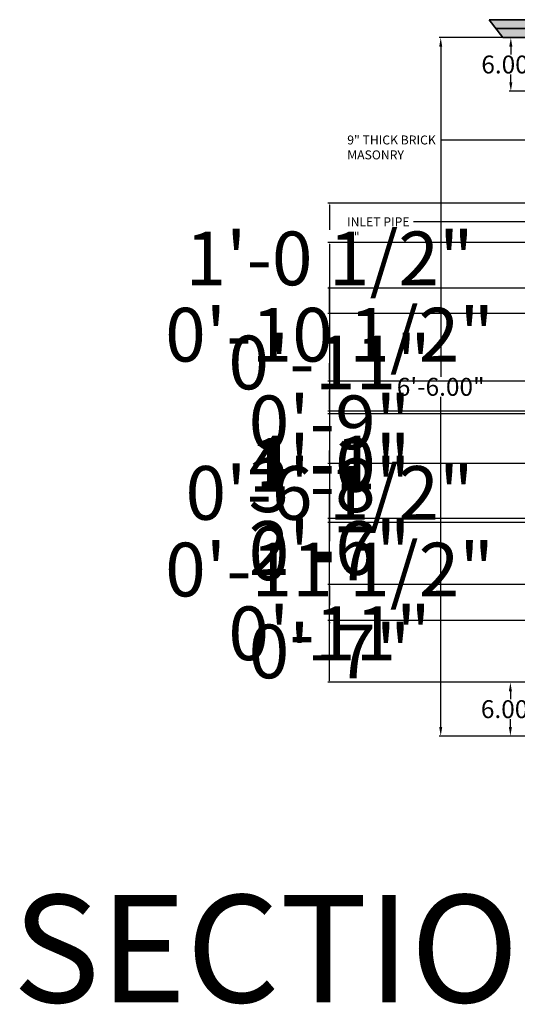
# Model space of a CAD drawing. Units: inches. Extents: x -34 to 285, y -151 to 155.
# Tile 1 of 10: x -34 to 22, y -151 to -41. Entities that reach past the tile are written whole.
import ezdxf
from ezdxf import colors
from ezdxf.entities.mleader import LeaderData, LeaderLine
from ezdxf.math import Vec2, Vec3

# ---------------------------------------------------------------- set-up
doc = ezdxf.new("R2010")
doc.units = ezdxf.units.IN
doc.header["$MEASUREMENT"] = 0
for name, color, linetype, lineweight in [('A-ANNO-DIMS', 2, 'Continuous', 18), ('A-ANNO-TEXT', 7, 'Continuous', 25), ('A-DETL', 7, 'Continuous', 35), ('A-DETL-PATT', 8, 'Continuous', 18)]:
    doc.layers.add(name, color=color, linetype=linetype, lineweight=lineweight)
doc.styles.get("Standard").update_dxf_attribs({"font": 'arial.ttf'})
doc.dimstyles.get("Standard").update_dxf_attribs({"dimtxt": 6, "dimasz": 0.18, "dimexe": 0.18, "dimexo": 0.0625, "dimgap": 0.09, "dimtad": 0, "dimtih": 1, "dimtoh": 1, "dimzin": 0, "dimdsep": 46, "dimlunit": 3, "dimtxsty": 'Standard', "dimcen": 0.09, "dimadec": 0, "dimazin": 0, "dimtfac": 1, "dimtofl": 0, "dimtmove": 0, "dimatfit": 3, "dimfxl": 1, "dimtolj": 1, "dimtzin": 0, "dimarcsym": 0})

# ---------------------------------------------------------------- blocks, each defined once
blk = doc.blocks.new('*D35')
at = {"layer": 'A-ANNO-DIMS', "color": 0, "lineweight": -2, "transparency": 16777216}
for p, q in [((21.5, -42.97), (13.14, -42.97)), ((13.32, -43.97), (13.32, -80.86)), ((13.32, -119.97), (13.32, -83.08)), ((22.78, -120.97), (13.14, -120.97))]:
    blk.add_line(p, q, dxfattribs=at)
at = {"layer": 'A-ANNO-DIMS', "color": 0, "transparency": 16777216}
for points in [[(13.16, -43.97), (13.49, -43.97), (13.32, -42.97)], [(13.16, -119.97), (13.49, -119.97), (13.32, -120.97)]]:
    blk.add_solid(points, dxfattribs=at)
at = {"layer": 'Defpoints', "color": 0, "transparency": 16777216}
for p in [(13.32, -42.97), (21.56, -42.97), (22.85, -120.97)]:
    blk.add_point(p, dxfattribs=at)
at = {"layer": 'A-ANNO-DIMS', "color": 0, "transparency": 16777216, "insert": (13.32, -81.97), "char_height": 2, "attachment_point": 5}
blk.add_mtext('\\A1;6\'-6.00"', dxfattribs=at)
blk = doc.blocks.new('*D36')
at = {"layer": 'A-ANNO-DIMS', "color": 0, "lineweight": -2, "transparency": 16777216}
for p, q in [((22.78, -42.97), (20.98, -42.97)), ((21.16, -43.97), (21.16, -44.86)), ((21.16, -47.97), (21.16, -47.08)), ((22.78, -48.97), (20.98, -48.97))]:
    blk.add_line(p, q, dxfattribs=at)
at = {"layer": 'A-ANNO-DIMS', "color": 0, "transparency": 16777216}
for points in [[(20.99, -43.97), (21.33, -43.97), (21.16, -42.97)], [(20.99, -47.97), (21.33, -47.97), (21.16, -48.97)]]:
    blk.add_solid(points, dxfattribs=at)
at = {"layer": 'Defpoints', "color": 0, "transparency": 16777216}
for p in [(22.85, -42.97), (21.16, -48.97), (22.85, -48.97)]:
    blk.add_point(p, dxfattribs=at)
at = {"layer": 'A-ANNO-DIMS', "color": 0, "transparency": 16777216, "insert": (21.16, -45.97), "char_height": 2, "attachment_point": 5}
blk.add_mtext('\\A1;6.00"', dxfattribs=at)
blk = doc.blocks.new('*D37')
at = {"layer": 'A-ANNO-DIMS', "color": 0, "lineweight": -2, "transparency": 16777216}
for p, q in [((22.78, -114.97), (20.93, -114.97)), ((21.11, -115.97), (21.11, -116.86)), ((21.11, -119.97), (21.11, -119.08)), ((22.78, -120.97), (20.93, -120.97))]:
    blk.add_line(p, q, dxfattribs=at)
at = {"layer": 'A-ANNO-DIMS', "color": 0, "transparency": 16777216}
for points in [[(20.94, -115.97), (21.28, -115.97), (21.11, -114.97)], [(20.94, -119.97), (21.28, -119.97), (21.11, -120.97)]]:
    blk.add_solid(points, dxfattribs=at)
at = {"layer": 'Defpoints', "color": 0, "transparency": 16777216}
for p in [(22.85, -114.97), (21.11, -120.97), (22.85, -120.97)]:
    blk.add_point(p, dxfattribs=at)
at = {"layer": 'A-ANNO-DIMS', "color": 0, "transparency": 16777216, "insert": (21.11, -117.97), "char_height": 2, "attachment_point": 5}
blk.add_mtext('\\A1;6.00"', dxfattribs=at)
blk = doc.blocks.new('*D57')
at = {"layer": 'A-ANNO-DIMS', "color": 0, "lineweight": -2, "transparency": 16777216}
for p, q in [((41.32, -65.85), (0.72, -65.85)), ((0.9, -66.03), (0.9, -87.31)), ((0.9, -114.79), (0.9, -93.51)), ((40.78, -114.97), (0.72, -114.97))]:
    blk.add_line(p, q, dxfattribs=at)
at = {"layer": 'A-ANNO-DIMS', "color": 0, "transparency": 16777216}
for points in [[(0.87, -66.03), (0.93, -66.03), (0.9, -65.85)], [(0.87, -114.79), (0.93, -114.79), (0.9, -114.97)]]:
    blk.add_solid(points, dxfattribs=at)
at = {"layer": 'Defpoints', "color": 0, "transparency": 16777216}
for p in [(41.38, -65.85), (0.9, -114.97), (40.85, -114.97)]:
    blk.add_point(p, dxfattribs=at)
at = {"layer": 'A-ANNO-DIMS', "color": 0, "transparency": 16777216, "insert": (0.9, -90.41), "char_height": 6, "attachment_point": 5}
blk.add_mtext('\\A1;4\'-1"', dxfattribs=at)
blk = doc.blocks.new('*D64')
at = {"layer": 'A-ANNO-DIMS', "color": 0, "lineweight": -2, "transparency": 16777216}
for p, q in [((157.78, -84.97), (0.72, -84.97)), ((0.9, -85.15), (0.9, -96.82)), ((0.9, -114.79), (0.9, -103.12)), ((148.78, -114.97), (0.72, -114.97))]:
    blk.add_line(p, q, dxfattribs=at)
at = {"layer": 'A-ANNO-DIMS', "color": 0, "transparency": 16777216}
for points in [[(0.87, -85.15), (0.93, -85.15), (0.9, -84.97)], [(0.87, -114.79), (0.93, -114.79), (0.9, -114.97)]]:
    blk.add_solid(points, dxfattribs=at)
at = {"layer": 'Defpoints', "color": 0, "transparency": 16777216}
for p in [(157.85, -84.97), (0.9, -114.97), (148.85, -114.97)]:
    blk.add_point(p, dxfattribs=at)
at = {"layer": 'A-ANNO-DIMS', "color": 0, "transparency": 16777216, "insert": (0.9, -99.97), "char_height": 6, "attachment_point": 5}
blk.add_mtext('\\A1;2\'-6"', dxfattribs=at)
blk = doc.blocks.new('*D67')
at = {"layer": 'A-ANNO-DIMS', "color": 0, "lineweight": -2, "transparency": 16777216}
for p, q in [((90.32, -70.95), (0.72, -70.95)), ((0.9, -71.13), (0.9, -89.8)), ((0.9, -114.79), (0.9, -96.11)), ((118.78, -114.97), (0.72, -114.97))]:
    blk.add_line(p, q, dxfattribs=at)
at = {"layer": 'A-ANNO-DIMS', "color": 0, "transparency": 16777216}
for points in [[(0.87, -71.13), (0.93, -71.13), (0.9, -70.95)], [(0.87, -114.79), (0.93, -114.79), (0.9, -114.97)]]:
    blk.add_solid(points, dxfattribs=at)
at = {"layer": 'Defpoints', "color": 0, "transparency": 16777216}
for p in [(90.38, -70.95), (0.9, -114.97), (118.85, -114.97)]:
    blk.add_point(p, dxfattribs=at)
at = {"layer": 'A-ANNO-DIMS', "color": 0, "transparency": 16777216, "insert": (0.9, -92.96), "char_height": 6, "attachment_point": 5}
blk.add_mtext('\\A1;3\'-8"', dxfattribs=at)
blk = doc.blocks.new('*D72')
at = {"layer": 'A-ANNO-DIMS', "color": 0, "lineweight": -2, "transparency": 16777216}
for p, q in [((90.32, -70.95), (0.72, -70.95)), ((0.9, -71.13), (0.9, -72.95)), ((0.9, -81.16), (0.9, -79.34)), ((97.61, -81.34), (0.72, -81.34))]:
    blk.add_line(p, q, dxfattribs=at)
at = {"layer": 'A-ANNO-DIMS', "color": 0, "transparency": 16777216}
for points in [[(0.87, -71.13), (0.93, -71.13), (0.9, -70.95)], [(0.87, -81.16), (0.93, -81.16), (0.9, -81.34)]]:
    blk.add_solid(points, dxfattribs=at)
at = {"layer": 'Defpoints', "color": 0, "transparency": 16777216}
for p in [(90.38, -70.95), (0.9, -81.34), (97.67, -81.34)]:
    blk.add_point(p, dxfattribs=at)
at = {"layer": 'A-ANNO-DIMS', "color": 0, "transparency": 16777216, "insert": (0.9, -76.15), "char_height": 6, "attachment_point": 5}
blk.add_mtext('\\A1;0\'-10 1/2"', dxfattribs=at)
blk = doc.blocks.new('*D73')
at = {"layer": 'A-ANNO-DIMS', "color": 0, "lineweight": -2, "transparency": 16777216}
for p, q in [((97.61, -81.34), (0.72, -81.34)), ((0.9, -81.52), (0.9, -82.78)), ((0.9, -90.35), (0.9, -89.09)), ((105.24, -90.53), (0.72, -90.53))]:
    blk.add_line(p, q, dxfattribs=at)
at = {"layer": 'A-ANNO-DIMS', "color": 0, "transparency": 16777216}
for points in [[(0.87, -81.52), (0.93, -81.52), (0.9, -81.34)], [(0.87, -90.35), (0.93, -90.35), (0.9, -90.53)]]:
    blk.add_solid(points, dxfattribs=at)
at = {"layer": 'Defpoints', "color": 0, "transparency": 16777216}
for p in [(97.67, -81.34), (0.9, -90.53), (105.3, -90.53)]:
    blk.add_point(p, dxfattribs=at)
at = {"layer": 'A-ANNO-DIMS', "color": 0, "transparency": 16777216, "insert": (0.9, -85.94), "char_height": 6, "attachment_point": 5}
blk.add_mtext('\\A1;0\'-9"', dxfattribs=at)
blk = doc.blocks.new('*D74')
at = {"layer": 'A-ANNO-DIMS', "color": 0, "lineweight": -2, "transparency": 16777216}
for p, q in [((0.9, -90.35), (0.9, -90.17)), ((105.24, -90.53), (0.72, -90.53)), ((115.99, -97.12), (0.72, -97.12)), ((0.9, -97.3), (0.9, -97.48))]:
    blk.add_line(p, q, dxfattribs=at)
at = {"layer": 'A-ANNO-DIMS', "color": 0, "transparency": 16777216}
for points in [[(0.87, -90.35), (0.93, -90.35), (0.9, -90.53)], [(0.87, -97.3), (0.93, -97.3), (0.9, -97.12)]]:
    blk.add_solid(points, dxfattribs=at)
at = {"layer": 'Defpoints', "color": 0, "transparency": 16777216}
for p in [(105.3, -90.53), (0.9, -97.12), (116.05, -97.12)]:
    blk.add_point(p, dxfattribs=at)
at = {"layer": 'A-ANNO-DIMS', "color": 0, "transparency": 16777216, "insert": (0.9, -93.82), "char_height": 6, "attachment_point": 5}
blk.add_mtext('\\A1;0\'-6 1/2"', dxfattribs=at)
blk = doc.blocks.new('*D75')
at = {"layer": 'A-ANNO-DIMS', "color": 0, "lineweight": -2, "transparency": 16777216}
for p, q in [((115.99, -97.12), (0.72, -97.12)), ((0.9, -97.3), (0.9, -97.42)), ((121.84, -104.03), (0.72, -104.03)), ((0.9, -103.85), (0.9, -103.73))]:
    blk.add_line(p, q, dxfattribs=at)
at = {"layer": 'A-ANNO-DIMS', "color": 0, "transparency": 16777216}
for points in [[(0.87, -97.3), (0.93, -97.3), (0.9, -97.12)], [(0.87, -103.85), (0.93, -103.85), (0.9, -104.03)]]:
    blk.add_solid(points, dxfattribs=at)
at = {"layer": 'Defpoints', "color": 0, "transparency": 16777216}
for p in [(116.05, -97.12), (0.9, -104.03), (121.9, -104.03)]:
    blk.add_point(p, dxfattribs=at)
at = {"layer": 'A-ANNO-DIMS', "color": 0, "transparency": 16777216, "insert": (0.9, -100.57), "char_height": 6, "attachment_point": 5}
blk.add_mtext('\\A1;0\'-7"', dxfattribs=at)
blk = doc.blocks.new('*D76')
at = {"layer": 'A-ANNO-DIMS', "color": 0, "lineweight": -2, "transparency": 16777216}
for p, q in [((121.84, -104.03), (0.72, -104.03)), ((0.9, -104.21), (0.9, -106.35)), ((0.9, -114.79), (0.9, -112.65)), ((118.78, -114.97), (0.72, -114.97))]:
    blk.add_line(p, q, dxfattribs=at)
at = {"layer": 'A-ANNO-DIMS', "color": 0, "transparency": 16777216}
for points in [[(0.87, -104.21), (0.93, -104.21), (0.9, -104.03)], [(0.87, -114.79), (0.93, -114.79), (0.9, -114.97)]]:
    blk.add_solid(points, dxfattribs=at)
at = {"layer": 'Defpoints', "color": 0, "transparency": 16777216}
for p in [(121.9, -104.03), (0.9, -114.97), (118.85, -114.97)]:
    blk.add_point(p, dxfattribs=at)
at = {"layer": 'A-ANNO-DIMS', "color": 0, "transparency": 16777216, "insert": (0.9, -109.5), "char_height": 6, "attachment_point": 5}
blk.add_mtext('\\A1;0\'-11"', dxfattribs=at)
blk = doc.blocks.new('*D83')
at = {"layer": 'A-ANNO-DIMS', "color": 0, "lineweight": -2, "transparency": 16777216}
for p, q in [((153.65, -61.45), (0.72, -61.45)), ((0.9, -61.63), (0.9, -64.43)), ((0.9, -73.62), (0.9, -70.82)), ((162.65, -73.8), (0.72, -73.8))]:
    blk.add_line(p, q, dxfattribs=at)
at = {"layer": 'A-ANNO-DIMS', "color": 0, "transparency": 16777216}
for points in [[(0.87, -61.63), (0.93, -61.63), (0.9, -61.45)], [(0.87, -73.62), (0.93, -73.62), (0.9, -73.8)]]:
    blk.add_solid(points, dxfattribs=at)
at = {"layer": 'Defpoints', "color": 0, "transparency": 16777216}
for p in [(153.71, -61.45), (0.9, -73.8), (162.71, -73.8)]:
    blk.add_point(p, dxfattribs=at)
at = {"layer": 'A-ANNO-DIMS', "color": 0, "transparency": 16777216, "insert": (0.9, -67.63), "char_height": 6, "attachment_point": 5}
blk.add_mtext('\\A1;1\'-0 1/2"', dxfattribs=at)
blk = doc.blocks.new('*D84')
at = {"layer": 'A-ANNO-DIMS', "color": 0, "lineweight": -2, "transparency": 16777216}
for p, q in [((162.65, -73.8), (0.72, -73.8)), ((0.9, -73.98), (0.9, -76.09)), ((0.9, -84.51), (0.9, -82.4)), ((169.24, -84.69), (0.72, -84.69))]:
    blk.add_line(p, q, dxfattribs=at)
at = {"layer": 'A-ANNO-DIMS', "color": 0, "transparency": 16777216}
for points in [[(0.87, -73.98), (0.93, -73.98), (0.9, -73.8)], [(0.87, -84.51), (0.93, -84.51), (0.9, -84.69)]]:
    blk.add_solid(points, dxfattribs=at)
at = {"layer": 'Defpoints', "color": 0, "transparency": 16777216}
for p in [(162.71, -73.8), (0.9, -84.69), (169.3, -84.69)]:
    blk.add_point(p, dxfattribs=at)
at = {"layer": 'A-ANNO-DIMS', "color": 0, "transparency": 16777216, "insert": (0.9, -79.25), "char_height": 6, "attachment_point": 5}
blk.add_mtext('\\A1;0\'-11"', dxfattribs=at)
blk = doc.blocks.new('*D85')
at = {"layer": 'A-ANNO-DIMS', "color": 0, "lineweight": -2, "transparency": 16777216}
for p, q in [((169.24, -84.69), (0.72, -84.69)), ((0.9, -84.87), (0.9, -87.54)), ((0.9, -96.51), (0.9, -93.85)), ((179.42, -96.69), (0.72, -96.69))]:
    blk.add_line(p, q, dxfattribs=at)
at = {"layer": 'A-ANNO-DIMS', "color": 0, "transparency": 16777216}
for points in [[(0.87, -84.87), (0.93, -84.87), (0.9, -84.69)], [(0.87, -96.51), (0.93, -96.51), (0.9, -96.69)]]:
    blk.add_solid(points, dxfattribs=at)
at = {"layer": 'Defpoints', "color": 0, "transparency": 16777216}
for p in [(169.3, -84.69), (0.9, -96.69), (179.48, -96.69)]:
    blk.add_point(p, dxfattribs=at)
at = {"layer": 'A-ANNO-DIMS', "color": 0, "transparency": 16777216, "insert": (0.9, -90.69), "char_height": 6, "attachment_point": 5}
blk.add_mtext('\\A1;1\'-0"', dxfattribs=at)
blk = doc.blocks.new('*D86')
at = {"layer": 'A-ANNO-DIMS', "color": 0, "lineweight": -2, "transparency": 16777216}
for p, q in [((179.42, -96.69), (0.72, -96.69)), ((0.9, -96.87), (0.9, -99.19)), ((0.9, -107.89), (0.9, -105.57)), ((187.78, -108.07), (0.72, -108.07))]:
    blk.add_line(p, q, dxfattribs=at)
at = {"layer": 'A-ANNO-DIMS', "color": 0, "transparency": 16777216}
for points in [[(0.87, -96.87), (0.93, -96.87), (0.9, -96.69)], [(0.87, -107.89), (0.93, -107.89), (0.9, -108.07)]]:
    blk.add_solid(points, dxfattribs=at)
at = {"layer": 'Defpoints', "color": 0, "transparency": 16777216}
for p in [(179.48, -96.69), (0.9, -108.07), (187.85, -108.07)]:
    blk.add_point(p, dxfattribs=at)
at = {"layer": 'A-ANNO-DIMS', "color": 0, "transparency": 16777216, "insert": (0.9, -102.38), "char_height": 6, "attachment_point": 5}
blk.add_mtext('\\A1;0\'-11 1/2"', dxfattribs=at)
blk = doc.blocks.new('*D87')
at = {"layer": 'A-ANNO-DIMS', "color": 0, "lineweight": -2, "transparency": 16777216}
for p, q in [((187.78, -108.07), (0.72, -108.07)), ((0.9, -108.25), (0.9, -108.37)), ((196.78, -114.97), (0.72, -114.97)), ((0.9, -114.79), (0.9, -114.67))]:
    blk.add_line(p, q, dxfattribs=at)
at = {"layer": 'A-ANNO-DIMS', "color": 0, "transparency": 16777216}
for points in [[(0.87, -108.25), (0.93, -108.25), (0.9, -108.07)], [(0.87, -114.79), (0.93, -114.79), (0.9, -114.97)]]:
    blk.add_solid(points, dxfattribs=at)
at = {"layer": 'Defpoints', "color": 0, "transparency": 16777216}
for p in [(187.85, -108.07), (0.9, -114.97), (196.85, -114.97)]:
    blk.add_point(p, dxfattribs=at)
at = {"layer": 'A-ANNO-DIMS', "color": 0, "transparency": 16777216, "insert": (0.9, -111.52), "char_height": 6, "attachment_point": 5}
blk.add_mtext('\\A1;0\'-7"', dxfattribs=at)

msp = doc.modelspace()

# ---------------------------------------------------------------- hatches: boundary and pattern name
at = {"layer": 'A-DETL-PATT'}
h = msp.add_hatch(dxfattribs=at)
h.set_pattern_fill('AR-SAND', color=256, scale=0.1)
h.paths.add_polyline_path([(43.43, -40.969), (20.939, -40.969), (18.752, -40.969), (19.516, -41.969), (43.43, -41.969)])
h.paths.add_polyline_path([(43.43, -41.969), (19.516, -41.969), (20.279, -42.969), (22.846, -42.969), (43.43, -42.969)])

# ---------------------------------------------------------------- linework, layer by layer
at = {"layer": 'A-DETL'}
for p, q in [((20.939, -40.969), (18.752, -40.969)), ((18.752, -40.969), (20.279, -42.969)), ((20.939, -40.969), (43.43, -40.969)), ((19.516, -41.969), (43.43, -41.969)), ((22.846, -42.969), (20.279, -42.969))]:
    msp.add_line(p, q, dxfattribs=at)

# ---------------------------------------------------------------- texts
at = {"layer": 'A-ANNO-TEXT', "insert": (-34.52, -138.72), "char_height": 12, "attachment_point": 1}
msp.add_mtext_dynamic_manual_height_columns('SECTIONAL ELEVATION OF A SEPTIC TANK ', width=509.35271, gutter_width=1, heights=[0], dxfattribs=at)

# ---------------------------------------------------------------- dimensions: what is measured, and where the dimension line sits
at = {"layer": 'A-ANNO-DIMS'}
for base, p1, p2, override, picture, middle in [((13.324, -42.969), (22.846, -120.969), (21.563, -42.969), {"dimtxt": 2, "dimasz": 1, "dimclrd": 0, "dimclre": 0, "dimclrt": 0}, '*D35', (13.324, -81.969)), ((21.161, -48.969), (22.846, -42.969), (22.846, -48.969), {"dimtxt": 2, "dimasz": 1, "dimclrd": 0, "dimclre": 0, "dimclrt": 0}, '*D36', (21.161, -45.969)), ((0.902, -73.803), (153.715, -61.451), (162.715, -73.803), {"dimdec": 1, "dimlfac": 1, "dimrnd": 0, "dimzin": 1, "dimdsep": 46, "dimlunit": 4, "dimfrac": 2}, '*D83', (0.902, -67.627)), ((0.902, -114.969), (41.384, -65.853), (40.846, -114.969), {"dimdec": 1, "dimlfac": 1, "dimrnd": 0, "dimzin": 1, "dimdsep": 46, "dimlunit": 4, "dimfrac": 2}, '*D57', (0.902, -90.411)), ((0.902, -81.345), (90.383, -70.947), (97.668, -81.345), {"dimdec": 1, "dimlfac": 1, "dimrnd": 0, "dimzin": 1, "dimdsep": 46, "dimlunit": 4, "dimfrac": 2}, '*D72', (0.902, -76.146)), ((0.902, -114.969), (90.383, -70.947), (118.846, -114.969), {"dimdec": 1, "dimlfac": 1, "dimrnd": 0, "dimzin": 1, "dimdsep": 46, "dimlunit": 4, "dimfrac": 2}, '*D67', (0.902, -92.958)), ((0.902, -84.693), (162.715, -73.803), (169.303, -84.693), {"dimdec": 1, "dimlfac": 1, "dimrnd": 0, "dimzin": 1, "dimdsep": 46, "dimlunit": 4, "dimfrac": 2}, '*D84', (0.902, -79.248)), ((0.902, -90.53), (97.668, -81.345), (105.299, -90.53), {"dimdec": 1, "dimlfac": 1, "dimrnd": 0, "dimzin": 1, "dimdsep": 46, "dimlunit": 4, "dimfrac": 2}, '*D73', (0.902, -85.937)), ((0.902, -97.116), (105.299, -90.53), (116.051, -97.116), {"dimdec": 1, "dimlfac": 1, "dimrnd": 0, "dimzin": 1, "dimdsep": 46, "dimlunit": 4, "dimfrac": 2}, '*D74', (0.902, -93.823)), ((0.902, -96.693), (169.303, -84.693), (179.482, -96.693), {"dimdec": 1, "dimlfac": 1, "dimrnd": 0, "dimzin": 1, "dimdsep": 46, "dimlunit": 4, "dimfrac": 2}, '*D85', (0.902, -90.693)), ((0.902, -114.969), (157.846, -84.969), (148.846, -114.969), {"dimdec": 1, "dimlfac": 1, "dimrnd": 0, "dimzin": 1, "dimdsep": 46, "dimlunit": 4, "dimfrac": 2}, '*D64', (0.902, -99.969)), ((0.902, -108.07), (179.482, -96.693), (187.846, -108.07), {"dimdec": 1, "dimlfac": 1, "dimrnd": 0, "dimzin": 1, "dimdsep": 46, "dimlunit": 4, "dimfrac": 2}, '*D86', (0.902, -102.381)), ((0.902, -104.028), (116.051, -97.116), (121.899, -104.028), {"dimdec": 1, "dimlfac": 1, "dimrnd": 0, "dimzin": 1, "dimdsep": 46, "dimlunit": 4, "dimfrac": 2}, '*D75', (0.902, -100.572)), ((0.902, -114.969), (121.899, -104.028), (118.846, -114.969), {"dimdec": 1, "dimlfac": 1, "dimrnd": 0, "dimzin": 1, "dimdsep": 46, "dimlunit": 4, "dimfrac": 2}, '*D76', (0.902, -109.499)), ((0.902, -114.969), (187.846, -108.07), (196.846, -114.969), {"dimdec": 1, "dimlfac": 1, "dimrnd": 0, "dimzin": 1, "dimdsep": 46, "dimlunit": 4, "dimfrac": 2}, '*D87', (0.902, -111.519)), ((21.111, -120.969), (22.846, -114.969), (22.846, -120.969), {"dimtxt": 2, "dimasz": 1, "dimclrd": 0, "dimclre": 0, "dimclrt": 0}, '*D37', (21.111, -117.969))]:
    dim = msp.add_linear_dim(base=base, p1=p1, p2=p2, angle=90, dimstyle='Standard', override=override, dxfattribs=at)
    dim.commit()
    dim.dimension.update_dxf_attribs({"geometry": picture, "text_midpoint": middle})

# ---------------------------------------------------------------- leaders
at = {"layer": 'A-ANNO-TEXT'}
ml = msp.add_multileader_mtext('Standard', dxfattribs=at)
ml.set_content('9" THICK BRICK \\PMASONRY ', color=(248, 215, 49))
ml.set_leader_properties()
ml.build(insert=Vec2(0, 0))
ml.multileader.update_dxf_attribs({"dogleg_length": 4.22, "arrow_head_size": 3})
ctx = ml.context
ctx.base_point, ctx.char_height, ctx.arrow_head_size, ctx.landing_gap_size, ctx.plane_origin = Vec3(2.785, -54.411), 1, 3, 0.09, Vec3(31.846, -54.411)
notes = []
notes.append((ctx, [(0, (1, 1, 0), (17.634, -54.411), (-1, 0), 4.22, [(0, [(31.846, -54.411)], 0, [])])]))
ctx.mtext.insert, ctx.mtext.flow_direction = Vec3(2.875, -53.902), 5
ml = msp.add_multileader_mtext('Standard', dxfattribs=at)
ml.set_content('INLET PIPE\\P4" ', color=(248, 215, 49))
ml.set_leader_properties()
ml.build(insert=Vec2(0, 0))
ml.multileader.update_dxf_attribs({"dogleg_length": 4.22, "arrow_head_size": 3})
ctx = ml.context
ctx.base_point, ctx.char_height, ctx.arrow_head_size, ctx.landing_gap_size, ctx.plane_origin = Vec3(2.763, -63.539), 1, 3, 0.09, Vec3(34.669, -63.539)
notes.append((ctx, [(0, (1, 1, 0), (14.489, -63.539), (-1, 0), 4.22, [(0, [(34.669, -63.539)], 0, [])])]))
ctx.mtext.insert, ctx.mtext.flow_direction = Vec3(2.853, -63.039), 5
for ctx, leaders in notes:
    for number, flags, end, landing, length, lines in leaders:
        leader = LeaderData()
        leader.index, (leader.has_last_leader_line, leader.has_dogleg_vector, leader.attachment_direction) = number, flags
        leader.last_leader_point, leader.dogleg_vector, leader.dogleg_length = Vec3(end), Vec3(landing), length
        for number, points, colour, breaks in lines:
            line = LeaderLine()
            line.index, line.vertices, line.color, line.breaks = number, Vec3.list(points), colors.encode_raw_color(colour), breaks
            leader.lines.append(line)
        ctx.leaders.append(leader)

doc.saveas('drawing.dxf')
